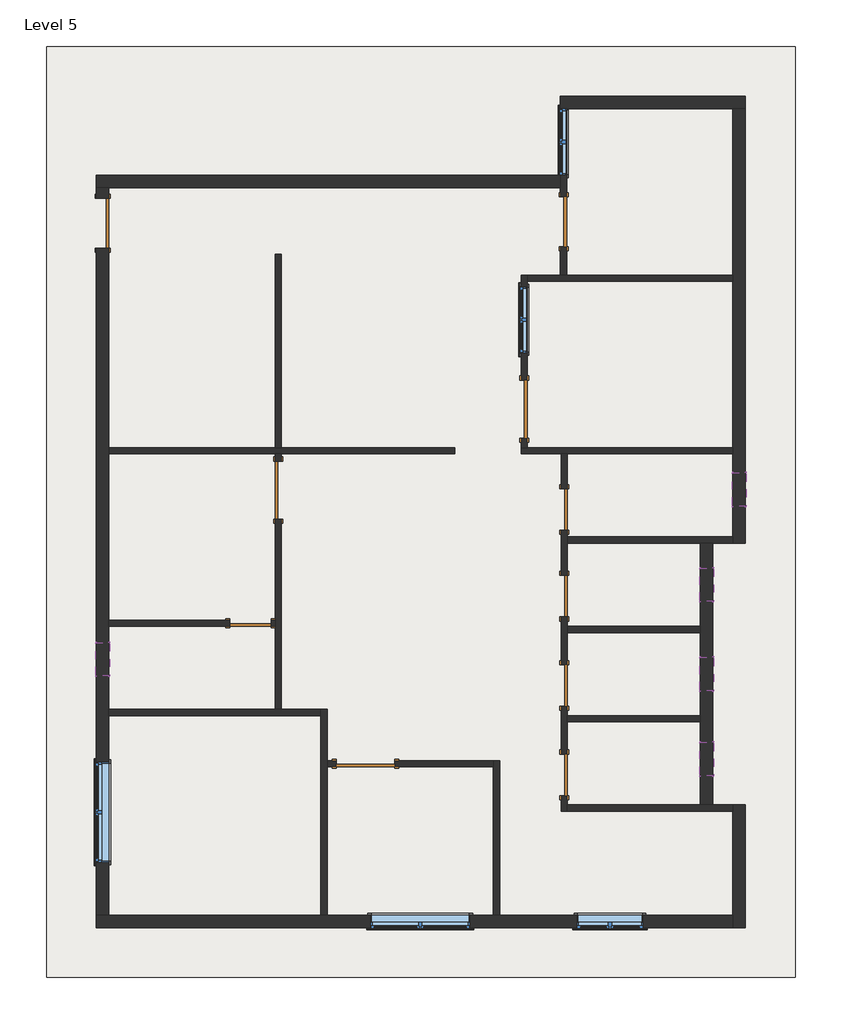
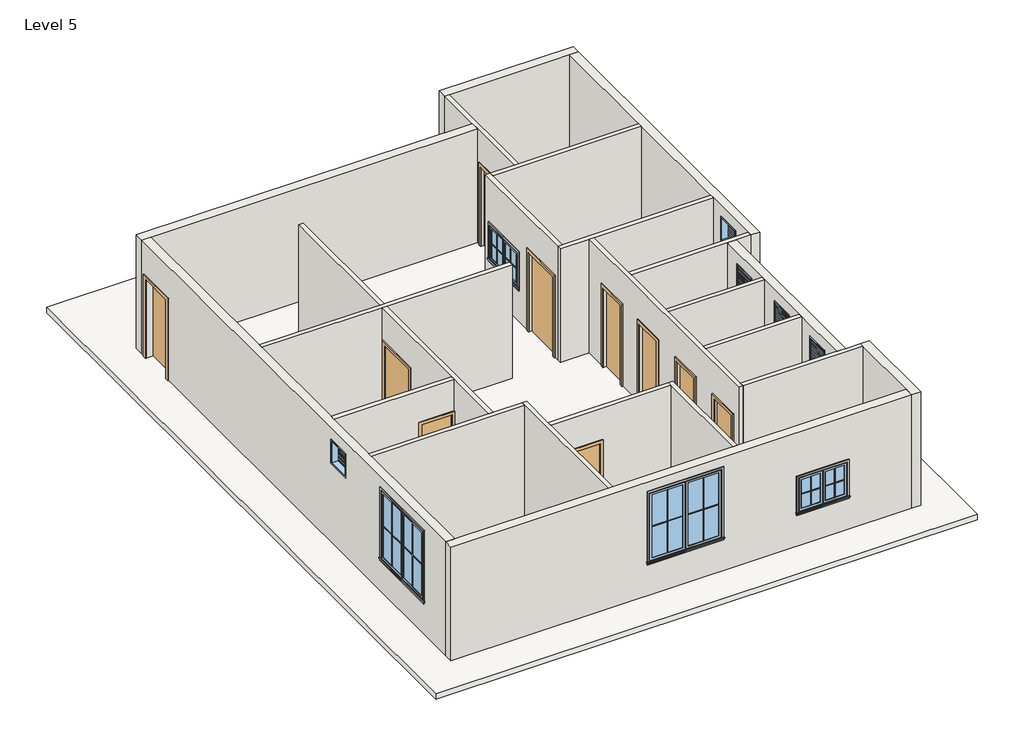
# One storey, incomplete: 23 walls, 20 proxies, 10 doors, 10 windows, 1 roof.
"""IFC4 building model written with IfcOpenShell, lengths in millimetres."""

from ifc_helpers import new_model, si_unit, frame, origin, place, context, project, spatial, polyline, outline, extrude, faceted_brep, transform, mapped, element, save
from components import muntin_pattern_2x2_muntin_pattern_2x2_0a037076, muntin_pattern_2x2_muntin_pattern_2x2_e6f69628, muntin_pattern_2x2_muntin_pattern_2x2_2357e71d, muntin_pattern_2x2_muntin_pattern_2x2_302d8f29, trim_window_exterior_flat_with_sill_b601e94a, trim_window_exterior_flat_with_sill_c4e67c73, trim_window_interior_flat_picture_frame_bfefb25c, trim_window_interior_flat_picture_frame_cf1733af, door_78caadf7, door_214872d5, single_flush_door_3_305aa2a5, single_flush_door_3_a90ba1ad, door_4c162e62, window_casement_double_win_4_c19c33cb, window_casement_double_win_4_2967420f, window_casement_double_win_6_ce442eab, window_f2d8fef0

model = new_model("IFC4")

# Units and contexts
model_context = context("Model", 3, world=origin())
ifc_project = project(units=[si_unit("LENGTHUNIT", "METRE", prefix="MILLI")], contexts=[model_context])

# Site, building, storey
site = spatial("IfcSite", under=ifc_project)
building = spatial("IfcBuilding", under=site)
storey = spatial("IfcBuildingStorey", under=building, Name="Level 5", Elevation=12649.2)

# Proxies
placement = place(None, origin())
muntin_pattern_2x2_muntin_pattern_2x2_shape = muntin_pattern_2x2_muntin_pattern_2x2_0a037076(model_context)
element("IfcBuildingElementProxy", 1, Name="Muntin Pattern_2x2 : Muntin Pattern_2x2", ObjectType="Muntin Pattern_2x2 : Muntin Pattern_2x2", at=placement, inside=storey, context=model_context, shape_type="MappedRepresentation", body=[
    mapped(muntin_pattern_2x2_muntin_pattern_2x2_shape, transform((-7058.058853, -4848.517381, 13633.45), x_axis=(0.0, 1.0, 0.0), y_axis=(-1.0, 0.0, 0.0), z_axis=(0.0, 0.0, 1.0))),
])
element("IfcBuildingElementProxy", 2, Name="Muntin Pattern_2x2 : Muntin Pattern_2x2", ObjectType="Muntin Pattern_2x2 : Muntin Pattern_2x2", at=placement, inside=storey, context=model_context, shape_type="MappedRepresentation", body=[
    mapped(muntin_pattern_2x2_muntin_pattern_2x2_shape, transform((-674.721353, -6497.929881, 13633.45), x_axis=(-1.0, 0.0, 0.0), y_axis=(0.0, -1.0, 0.0), z_axis=(0.0, 0.0, 1.0))),
])
muntin_pattern_2x2_muntin_pattern_2x2_2_shape = muntin_pattern_2x2_muntin_pattern_2x2_e6f69628(model_context)
element("IfcBuildingElementProxy", 3, Name="Muntin Pattern_2x2 : Muntin Pattern_2x2", ObjectType="Muntin Pattern_2x2 : Muntin Pattern_2x2", at=placement, inside=storey, context=model_context, shape_type="MappedRepresentation", body=[
    mapped(muntin_pattern_2x2_muntin_pattern_2x2_2_shape, transform((-7058.058853, -3937.292381, 13633.45), x_axis=(0.0, -1.0, 0.0), y_axis=(1.0, 0.0, 0.0), z_axis=(0.0, 0.0, 1.0))),
])
element("IfcBuildingElementProxy", 4, Name="Muntin Pattern_2x2 : Muntin Pattern_2x2", ObjectType="Muntin Pattern_2x2 : Muntin Pattern_2x2", at=placement, inside=storey, context=model_context, shape_type="MappedRepresentation", body=[
    mapped(muntin_pattern_2x2_muntin_pattern_2x2_2_shape, transform((-1585.946353, -6497.929881, 13633.45), x_axis=(1.0, 0.0, 0.0), y_axis=(0.0, 1.0, 0.0), z_axis=(0.0, 0.0, 1.0))),
])
muntin_pattern_2x2_muntin_pattern_2x2_3_shape = muntin_pattern_2x2_muntin_pattern_2x2_2357e71d(model_context)
element("IfcBuildingElementProxy", 5, Name="Muntin Pattern_2x2 : Muntin Pattern_2x2", ObjectType="Muntin Pattern_2x2 : Muntin Pattern_2x2", at=placement, inside=storey, context=model_context, shape_type="MappedRepresentation", body=[
    mapped(muntin_pattern_2x2_muntin_pattern_2x2_3_shape, transform((2652.678647, -6497.929881, 13633.45), x_axis=(-1.0, 0.0, 0.0), y_axis=(0.0, -1.0, 0.0), z_axis=(0.0, 0.0, 1.0))),
])
element("IfcBuildingElementProxy", 6, Name="Muntin Pattern_2x2 : Muntin Pattern_2x2", ObjectType="Muntin Pattern_2x2 : Muntin Pattern_2x2", at=placement, inside=storey, context=model_context, shape_type="MappedRepresentation", body=[
    mapped(muntin_pattern_2x2_muntin_pattern_2x2_3_shape, transform((727.041147, 4333.582619, 13633.45), x_axis=(0.0, 1.0, 0.0), y_axis=(-1.0, 0.0, 0.0), z_axis=(0.0, 0.0, 1.0))),
])
element("IfcBuildingElementProxy", 7, Name="Muntin Pattern_2x2 : Muntin Pattern_2x2", ObjectType="Muntin Pattern_2x2 : Muntin Pattern_2x2", at=placement, inside=storey, context=model_context, shape_type="MappedRepresentation", body=[
    mapped(muntin_pattern_2x2_muntin_pattern_2x2_3_shape, transform((1450.941147, 7591.132619, 13633.45), x_axis=(0.0, 1.0, 0.0), y_axis=(-1.0, 0.0, 0.0), z_axis=(0.0, 0.0, 1.0))),
])
muntin_pattern_2x2_muntin_pattern_2x2_4_shape = muntin_pattern_2x2_muntin_pattern_2x2_302d8f29(model_context)
element("IfcBuildingElementProxy", 8, Name="Muntin Pattern_2x2 : Muntin Pattern_2x2", ObjectType="Muntin Pattern_2x2 : Muntin Pattern_2x2", at=placement, inside=storey, context=model_context, shape_type="MappedRepresentation", body=[
    mapped(muntin_pattern_2x2_muntin_pattern_2x2_4_shape, transform((2046.253647, -6497.929881, 13633.45), x_axis=(1.0, 0.0, 0.0), y_axis=(0.0, 1.0, 0.0), z_axis=(0.0, 0.0, 1.0))),
])
element("IfcBuildingElementProxy", 9, Name="Muntin Pattern_2x2 : Muntin Pattern_2x2", ObjectType="Muntin Pattern_2x2 : Muntin Pattern_2x2", at=placement, inside=storey, context=model_context, shape_type="MappedRepresentation", body=[
    mapped(muntin_pattern_2x2_muntin_pattern_2x2_4_shape, transform((727.041147, 4940.007619, 13633.45), x_axis=(0.0, -1.0, 0.0), y_axis=(1.0, 0.0, 0.0), z_axis=(0.0, 0.0, 1.0))),
])
element("IfcBuildingElementProxy", 10, Name="Muntin Pattern_2x2 : Muntin Pattern_2x2", ObjectType="Muntin Pattern_2x2 : Muntin Pattern_2x2", at=placement, inside=storey, context=model_context, shape_type="MappedRepresentation", body=[
    mapped(muntin_pattern_2x2_muntin_pattern_2x2_4_shape, transform((1450.941147, 8197.557619, 13633.45), x_axis=(0.0, -1.0, 0.0), y_axis=(1.0, 0.0, 0.0), z_axis=(0.0, 0.0, 1.0))),
])
trim_window_exterior_flat_with_sill_shape = trim_window_exterior_flat_with_sill_b601e94a(model_context)
element("IfcBuildingElementProxy", 11, Name="Trim-Window-Exterior-Flat : with Sill", ObjectType="Trim-Window-Exterior-Flat : with Sill", at=placement, inside=storey, context=model_context, shape_type="MappedRepresentation", body=[
    mapped(trim_window_exterior_flat_with_sill_shape, transform((-7067.583853, -4392.904881, 15392.4), x_axis=(0.0, -1.0, 0.0), y_axis=(0.0, 0.0, 1.0), z_axis=(-1.0, 0.0, 0.0))),
])
element("IfcBuildingElementProxy", 12, Name="Trim-Window-Exterior-Flat : with Sill", ObjectType="Trim-Window-Exterior-Flat : with Sill", at=placement, inside=storey, context=model_context, shape_type="MappedRepresentation", body=[
    mapped(trim_window_exterior_flat_with_sill_shape, transform((-1130.333853, -6507.454881, 15392.4), x_axis=(1.0, 0.0, 0.0), y_axis=(0.0, 0.0, 1.0), z_axis=(0.0, -1.0, 0.0))),
])
trim_window_exterior_flat_with_sill_2_shape = trim_window_exterior_flat_with_sill_c4e67c73(model_context)
element("IfcBuildingElementProxy", 13, Name="Trim-Window-Exterior-Flat : with Sill", ObjectType="Trim-Window-Exterior-Flat : with Sill", at=placement, inside=storey, context=model_context, shape_type="MappedRepresentation", body=[
    mapped(trim_window_exterior_flat_with_sill_2_shape, transform((2349.466147, -6507.454881, 14478.0), x_axis=(1.0, 0.0, 0.0), y_axis=(0.0, 0.0, 1.0), z_axis=(0.0, -1.0, 0.0))),
])
element("IfcBuildingElementProxy", 14, Name="Trim-Window-Exterior-Flat : with Sill", ObjectType="Trim-Window-Exterior-Flat : with Sill", at=placement, inside=storey, context=model_context, shape_type="MappedRepresentation", body=[
    mapped(trim_window_exterior_flat_with_sill_2_shape, transform((717.516147, 4636.795119, 14478.0), x_axis=(0.0, -1.0, 0.0), y_axis=(0.0, 0.0, 1.0), z_axis=(-1.0, 0.0, 0.0))),
])
element("IfcBuildingElementProxy", 15, Name="Trim-Window-Exterior-Flat : with Sill", ObjectType="Trim-Window-Exterior-Flat : with Sill", at=placement, inside=storey, context=model_context, shape_type="MappedRepresentation", body=[
    mapped(trim_window_exterior_flat_with_sill_2_shape, transform((1441.416147, 7894.345119, 14478.0), x_axis=(0.0, -1.0, 0.0), y_axis=(0.0, 0.0, 1.0), z_axis=(-1.0, 0.0, 0.0))),
])
trim_window_interior_flat_picture_frame_shape = trim_window_interior_flat_picture_frame_bfefb25c(model_context)
element("IfcBuildingElementProxy", 16, Name="Trim-Window-Interior-Flat : Picture Frame", ObjectType="Trim-Window-Interior-Flat : Picture Frame", at=placement, inside=storey, context=model_context, shape_type="MappedRepresentation", body=[
    mapped(trim_window_interior_flat_picture_frame_shape, transform((-6838.983853, -4392.904881, 15392.4), x_axis=(0.0, 1.0, 0.0), y_axis=(0.0, 0.0, 1.0), z_axis=(1.0, 0.0, 0.0))),
])
element("IfcBuildingElementProxy", 17, Name="Trim-Window-Interior-Flat : Picture Frame", ObjectType="Trim-Window-Interior-Flat : Picture Frame", at=placement, inside=storey, context=model_context, shape_type="MappedRepresentation", body=[
    mapped(trim_window_interior_flat_picture_frame_shape, transform((-1130.333853, -6278.854881, 15392.4), x_axis=(-1.0, 0.0, 0.0), y_axis=(0.0, 0.0, 1.0), z_axis=(0.0, 1.0, 0.0))),
])
trim_window_interior_flat_picture_frame_2_shape = trim_window_interior_flat_picture_frame_cf1733af(model_context)
element("IfcBuildingElementProxy", 18, Name="Trim-Window-Interior-Flat : Picture Frame", ObjectType="Trim-Window-Interior-Flat : Picture Frame", at=placement, inside=storey, context=model_context, shape_type="MappedRepresentation", body=[
    mapped(trim_window_interior_flat_picture_frame_2_shape, transform((2349.466147, -6278.854881, 14478.0), x_axis=(-1.0, 0.0, 0.0), y_axis=(0.0, 0.0, 1.0), z_axis=(0.0, 1.0, 0.0))),
])
element("IfcBuildingElementProxy", 19, Name="Trim-Window-Interior-Flat : Picture Frame", ObjectType="Trim-Window-Interior-Flat : Picture Frame", at=placement, inside=storey, context=model_context, shape_type="MappedRepresentation", body=[
    mapped(trim_window_interior_flat_picture_frame_2_shape, transform((831.816147, 4636.795119, 14478.0), x_axis=(0.0, 1.0, 0.0), y_axis=(0.0, 0.0, 1.0), z_axis=(1.0, 0.0, 0.0))),
])
element("IfcBuildingElementProxy", 20, Name="Trim-Window-Interior-Flat : Picture Frame", ObjectType="Trim-Window-Interior-Flat : Picture Frame", at=placement, inside=storey, context=model_context, shape_type="MappedRepresentation", body=[
    mapped(trim_window_interior_flat_picture_frame_2_shape, transform((1555.716147, 7894.345119, 14478.0), x_axis=(0.0, 1.0, 0.0), y_axis=(0.0, 0.0, 1.0), z_axis=(1.0, 0.0, 0.0))),
])

# Doors
door_shape = door_78caadf7(model_context)
element("IfcDoor", 21, ObjectType="Single-Flush : 2'6\"", at=placement, inside=storey, context=model_context, shape_type="MappedRepresentation", body=[
    mapped(door_shape, transform((-4241.833853, -925.804881, 12649.2), x_axis=(1.0, 0.0, 0.0), y_axis=(0.0, 1.0, 0.0), z_axis=(0.0, 0.0, 1.0))),
])
door_2_shape = door_214872d5(model_context)
element("IfcDoor", 22, ObjectType="Single-Flush : 2'6\"", at=placement, inside=storey, context=model_context, shape_type="MappedRepresentation", body=[
    mapped(door_2_shape, transform((1511.266147, 1156.995119, 12649.2), x_axis=(0.0, -1.0, 0.0), y_axis=(1.0, 0.0, 0.0), z_axis=(0.0, 0.0, 1.0))),
])
element("IfcDoor", 23, ObjectType="Single-Flush : 2'6\"", at=placement, inside=storey, context=model_context, shape_type="MappedRepresentation", body=[
    mapped(door_2_shape, transform((1511.266147, -430.504881, 12649.2), x_axis=(0.0, -1.0, 0.0), y_axis=(1.0, 0.0, 0.0), z_axis=(0.0, 0.0, 1.0))),
])
element("IfcDoor", 24, ObjectType="Single-Flush : 2'6\"", at=placement, inside=storey, context=model_context, shape_type="MappedRepresentation", body=[
    mapped(door_2_shape, transform((1511.266147, -2068.804881, 12649.2), x_axis=(0.0, -1.0, 0.0), y_axis=(1.0, 0.0, 0.0), z_axis=(0.0, 0.0, 1.0))),
])
element("IfcDoor", 25, ObjectType="Single-Flush : 2'6\"", at=placement, inside=storey, context=model_context, shape_type="MappedRepresentation", body=[
    mapped(door_2_shape, transform((1511.266147, -3707.104881, 12649.2), x_axis=(0.0, -1.0, 0.0), y_axis=(1.0, 0.0, 0.0), z_axis=(0.0, 0.0, 1.0))),
])
single_flush_door_3_shape = single_flush_door_3_305aa2a5(model_context)
element("IfcDoor", 26, ObjectType="Single-Flush : DOOR 3'", at=placement, inside=storey, context=model_context, shape_type="MappedRepresentation", body=[
    mapped(single_flush_door_3_shape, transform((1498.566147, 6433.845119, 12649.2), x_axis=(0.0, 1.0, 0.0), y_axis=(-1.0, 0.0, 0.0), z_axis=(0.0, 0.0, 1.0))),
])
single_flush_door_3_2_shape = single_flush_door_3_a90ba1ad(model_context)
element("IfcDoor", 27, ObjectType="Single-Flush : DOOR 3'", at=placement, inside=storey, context=model_context, shape_type="MappedRepresentation", body=[
    mapped(single_flush_door_3_2_shape, transform((-6953.283853, 6408.445119, 12649.2), x_axis=(0.0, 1.0, 0.0), y_axis=(-1.0, 0.0, 0.0), z_axis=(0.0, 0.0, 1.0))),
])
door_3_shape = door_4c162e62(model_context)
element("IfcDoor", 28, ObjectType="Single-Flush : DOOR 3'6\"", at=placement, inside=storey, context=model_context, shape_type="MappedRepresentation", body=[
    mapped(door_3_shape, transform((-3733.833853, 1512.595119, 12649.2), x_axis=(0.0, 1.0, 0.0), y_axis=(-1.0, 0.0, 0.0), z_axis=(0.0, 0.0, 1.0))),
])
element("IfcDoor", 29, ObjectType="Single-Flush : DOOR 3'6\"", at=placement, inside=storey, context=model_context, shape_type="MappedRepresentation", body=[
    mapped(door_3_shape, transform((774.666147, 2998.495119, 12649.2), x_axis=(0.0, -1.0, 0.0), y_axis=(1.0, 0.0, 0.0), z_axis=(0.0, 0.0, 1.0))),
])
element("IfcDoor", 30, ObjectType="Single-Flush : DOOR 3'6\"", at=placement, inside=storey, context=model_context, shape_type="MappedRepresentation", body=[
    mapped(door_3_shape, transform((-2133.633853, -3503.904881, 12649.2), x_axis=(-1.0, 0.0, 0.0), y_axis=(0.0, -1.0, 0.0), z_axis=(0.0, 0.0, 1.0))),
])

# Roof
element("IfcRoof", 31, ObjectType="Generic - 12\"", at=placement, inside=storey, context=model_context, shape_type="SweptSolid", body=[
    extrude(outline(polyline([(-7981.983853, 9646.945119), (5746.716147, 9646.945119), (5746.716147, -7421.854881), (-7981.983853, -7421.854881), (-7981.983853, 9646.945119)])), frame((0.0, 0.0, 12496.8), z_axis=(0.0, 0.0, 1.0), x_axis=(1.0, 0.0, 0.0)), (0.0, 0.0, 1.0), 152.4),
])

# Walls
element("IfcWall", 32, ObjectType="WALL 4.5\"", at=placement, inside=storey, context=model_context, shape_type="Brep", body=[
    faceted_brep([(-6838.983853, 2179.345119, 12649.2), (-3790.983853, 2179.345119, 12649.2), (-3676.683853, 2179.345119, 12649.2), (-501.683853, 2179.345119, 12649.2), (-501.683853, 2179.345119, 15697.2), (-3676.683853, 2179.345119, 15697.2), (-3790.983853, 2179.345119, 15697.2), (-6838.983853, 2179.345119, 15697.2), (-6838.983853, 2293.645119, 12649.2), (-6838.983853, 2293.645119, 15697.2), (-3790.983853, 2293.645119, 15697.2), (-3676.683853, 2293.645119, 15697.2), (-501.683853, 2293.645119, 15697.2), (-501.683853, 2293.645119, 12649.2), (-3676.683853, 2293.645119, 12649.2), (-3790.983853, 2293.645119, 12649.2)], [[[0, 1, 2, 3, 4, 5, 6, 7]], [[8, 9, 10, 11, 12, 13, 14, 15]], [[3, 2, 1, 0, 8, 15, 14, 13]], [[4, 3, 13, 12]], [[0, 7, 9, 8]], [[7, 6, 5, 4, 12, 11, 10, 9]]]),
])
element("IfcWall", 33, ObjectType="WALL 4.5\"", at=placement, inside=storey, context=model_context, shape_type="Brep", body=[
    faceted_brep([(-2838.483853, -6278.854881, 12649.2), (-2838.483853, -3561.054881, 12649.2), (-2838.483853, -3446.754881, 12649.2), (-2838.483853, -2506.954881, 12649.2), (-2838.483853, -2506.954881, 15697.2), (-2838.483853, -3446.754881, 15697.2), (-2838.483853, -3561.054881, 15697.2), (-2838.483853, -6278.854881, 15697.2), (-2952.783853, -6278.854881, 12649.2), (-2952.783853, -6278.854881, 15697.2), (-2952.783853, -2621.254881, 15697.2), (-2952.783853, -2506.954881, 15697.2), (-2952.783853, -2506.954881, 12649.2), (-2952.783853, -2621.254881, 12649.2)], [[[0, 1, 2, 3, 4, 5, 6, 7]], [[8, 9, 10, 11, 12, 13]], [[3, 2, 1, 0, 8, 13, 12]], [[0, 7, 9, 8]], [[4, 3, 12, 11]], [[7, 6, 5, 4, 11, 10, 9]]]),
])
element("IfcWall", 34, ObjectType="WALL 4.5\"", at=placement, inside=storey, context=model_context, shape_type="Brep", body=[
    faceted_brep([(-2952.783853, -2506.954881, 12649.2), (-3676.683853, -2506.954881, 12649.2), (-3790.983853, -2506.954881, 12649.2), (-6838.983853, -2506.954881, 12649.2), (-6838.983853, -2506.954881, 15697.2), (-3790.983853, -2506.954881, 15697.2), (-3676.683853, -2506.954881, 15697.2), (-2952.783853, -2506.954881, 15697.2), (-2952.783853, -2621.254881, 12649.2), (-2952.783853, -2621.254881, 15697.2), (-6838.983853, -2621.254881, 15697.2), (-6838.983853, -2621.254881, 12649.2)], [[[0, 1, 2, 3, 4, 5, 6, 7]], [[8, 9, 10, 11]], [[3, 2, 1, 0, 8, 11]], [[0, 7, 9, 8]], [[4, 3, 11, 10]], [[7, 6, 5, 4, 10, 9]]]),
])
element("IfcWall", 35, ObjectType="WALL 4.5\"", at=placement, inside=storey, context=model_context, shape_type="SweptSolid", body=[
    extrude(outline(polyline([(14782.8, -3860.833853), (12649.2, -3860.833853), (12649.2, -3790.983853), (15697.2, -3790.983853), (15697.2, -6838.983853), (12649.2, -6838.983853), (12649.2, -4622.833853), (14782.8, -4622.833853), (14782.8, -3860.833853)])), frame((0.0, -982.954881, 0.0), z_axis=(0.0, 1.0, 0.0), x_axis=(0.0, 0.0, 1.0)), (0.0, 0.0, 1.0), 114.3),
])
element("IfcWall", 36, ObjectType="WALL 4.5\"", at=placement, inside=storey, context=model_context, shape_type="Brep", body=[
    faceted_brep([(-3676.683853, 5836.945119, 12649.2), (-3676.683853, 5836.945119, 15697.2), (-3676.683853, 2293.645119, 15697.2), (-3676.683853, 2293.645119, 12649.2), (-3790.983853, 5836.945119, 15697.2), (-3790.983853, 5836.945119, 12649.2), (-3790.983853, 2293.645119, 12649.2), (-3790.983853, 2293.645119, 15697.2)], [[[0, 1, 2, 3]], [[4, 5, 6, 7]], [[5, 0, 3, 6]], [[1, 0, 5, 4]], [[3, 2, 7, 6]], [[1, 4, 7, 2]]]),
    faceted_brep([(-3676.683853, -2506.954881, 15697.2), (-3676.683853, -2506.954881, 12649.2), (-3676.683853, 979.195119, 12649.2), (-3676.683853, 979.195119, 14782.8), (-3676.683853, 2045.995119, 14782.8), (-3676.683853, 2045.995119, 12649.2), (-3676.683853, 2179.345119, 12649.2), (-3676.683853, 2179.345119, 15697.2), (-3790.983853, -2506.954881, 12649.2), (-3790.983853, -2506.954881, 15697.2), (-3790.983853, -982.954881, 15697.2), (-3790.983853, -868.654881, 15697.2), (-3790.983853, 2179.345119, 15697.2), (-3790.983853, 2179.345119, 12649.2), (-3790.983853, 2045.995119, 12649.2), (-3790.983853, 2045.995119, 14782.8), (-3790.983853, 979.195119, 14782.8), (-3790.983853, 979.195119, 12649.2), (-3790.983853, -868.654881, 12649.2), (-3790.983853, -982.954881, 12649.2)], [[[0, 1, 2, 3, 4, 5, 6, 7]], [[8, 9, 10, 11, 12, 13, 14, 15, 16, 17, 18, 19]], [[1, 8, 19, 18, 17, 2]], [[5, 14, 13, 6]], [[1, 0, 9, 8]], [[7, 6, 13, 12]], [[15, 14, 5, 4]], [[16, 15, 4, 3]], [[17, 16, 3, 2]], [[9, 0, 7, 12, 11, 10]]]),
])
element("IfcWall", 37, ObjectType="WALL 4.5\"", at=placement, inside=storey, context=model_context, shape_type="Brep", body=[
    faceted_brep([(4603.716147, 2293.645119, 12649.2), (831.816147, 2293.645119, 12649.2), (717.516147, 2293.645119, 12649.2), (717.516147, 2293.645119, 15697.2), (831.816147, 2293.645119, 15697.2), (4603.716147, 2293.645119, 15697.2), (4603.716147, 2179.345119, 12649.2), (4603.716147, 2179.345119, 15697.2), (1568.416147, 2179.345119, 15697.2), (1454.116147, 2179.345119, 15697.2), (717.516147, 2179.345119, 15697.2), (717.516147, 2179.345119, 12649.2), (1454.116147, 2179.345119, 12649.2), (1568.416147, 2179.345119, 12649.2)], [[[0, 1, 2, 3, 4, 5]], [[6, 7, 8, 9, 10, 11, 12, 13]], [[2, 1, 0, 6, 13, 12, 11]], [[0, 5, 7, 6]], [[3, 2, 11, 10]], [[5, 4, 3, 10, 9, 8, 7]]]),
])
element("IfcWall", 38, ObjectType="WALL 4.5\"", at=placement, inside=storey, context=model_context, shape_type="Brep", body=[
    faceted_brep([(831.816147, 2293.645119, 12649.2), (831.816147, 2465.095119, 12649.2), (831.816147, 2465.095119, 14782.8), (831.816147, 3531.895119, 14782.8), (831.816147, 3531.895119, 12649.2), (831.816147, 5341.645119, 12649.2), (831.816147, 5455.945119, 12649.2), (831.816147, 5455.945119, 15697.2), (831.816147, 5341.645119, 15697.2), (831.816147, 2293.645119, 15697.2), (831.816147, 5246.395119, 14478.0), (831.816147, 5246.395119, 13563.6), (831.816147, 4027.195119, 13563.6), (831.816147, 4027.195119, 14478.0), (717.516147, 2465.095119, 14782.8), (717.516147, 2465.095119, 12649.2), (717.516147, 2293.645119, 12649.2), (717.516147, 2293.645119, 15697.2), (717.516147, 5455.945119, 15697.2), (717.516147, 5455.945119, 12649.2), (717.516147, 3531.895119, 12649.2), (717.516147, 3531.895119, 14782.8), (717.516147, 5246.395119, 14478.0), (717.516147, 4027.195119, 14478.0), (717.516147, 4027.195119, 13563.6), (717.516147, 5246.395119, 13563.6)], [[[0, 1, 2, 3, 4, 5, 6, 7, 8, 9], [10, 11, 12, 13]], [[14, 15, 16, 17, 18, 19, 20, 21], [22, 23, 24, 25]], [[20, 19, 6, 5, 4]], [[16, 15, 1, 0]], [[0, 9, 17, 16]], [[7, 6, 19, 18]], [[11, 10, 22, 25]], [[12, 11, 25, 24]], [[13, 12, 24, 23]], [[10, 13, 23, 22]], [[2, 1, 15, 14]], [[3, 2, 14, 21]], [[4, 3, 21, 20]], [[9, 8, 7, 18, 17]]]),
])
element("IfcWall", 39, ObjectType="WALL 4.5\"", at=placement, inside=storey, context=model_context, shape_type="Brep", body=[
    faceted_brep([(831.816147, 5341.645119, 12649.2), (4603.716147, 5341.645119, 12649.2), (4603.716147, 5341.645119, 15697.2), (831.816147, 5341.645119, 15697.2), (831.816147, 5455.945119, 12649.2), (831.816147, 5455.945119, 15697.2), (1441.416147, 5455.945119, 15697.2), (1555.716147, 5455.945119, 15697.2), (4603.716147, 5455.945119, 15697.2), (4603.716147, 5455.945119, 12649.2), (1555.716147, 5455.945119, 12649.2), (1441.416147, 5455.945119, 12649.2)], [[[0, 1, 2, 3]], [[4, 5, 6, 7, 8, 9, 10, 11]], [[1, 0, 4, 11, 10, 9]], [[0, 3, 5, 4]], [[2, 1, 9, 8]], [[3, 2, 8, 7, 6, 5]]]),
])
element("IfcWall", 40, ObjectType="WALL 4.5\"", at=placement, inside=storey, context=model_context, shape_type="Brep", body=[
    faceted_brep([(1555.716147, 6891.045119, 14782.8), (1555.716147, 6891.045119, 12649.2), (1555.716147, 8503.945119, 12649.2), (1555.716147, 8503.945119, 13563.6), (1555.716147, 7284.745119, 13563.6), (1555.716147, 7284.745119, 14478.0), (1555.716147, 8503.945119, 14478.0), (1555.716147, 8503.945119, 15697.2), (1555.716147, 5455.945119, 15697.2), (1555.716147, 5455.945119, 12649.2), (1555.716147, 5976.645119, 12649.2), (1555.716147, 5976.645119, 14782.8), (1441.416147, 8503.945119, 12649.2), (1441.416147, 7284.745119, 12649.2), (1441.416147, 7056.145119, 12649.2), (1441.416147, 6891.045119, 12649.2), (1441.416147, 6891.045119, 14782.8), (1441.416147, 5976.645119, 14782.8), (1441.416147, 5976.645119, 12649.2), (1441.416147, 5455.945119, 12649.2), (1441.416147, 5455.945119, 15697.2), (1441.416147, 7056.145119, 15697.2), (1441.416147, 7284.745119, 15697.2), (1441.416147, 8503.945119, 15697.2), (1441.416147, 8503.945119, 14478.0), (1441.416147, 7284.745119, 14478.0), (1441.416147, 7284.745119, 13563.6), (1441.416147, 8503.945119, 13563.6)], [[[0, 1, 2, 3, 4, 5, 6, 7, 8, 9, 10, 11]], [[12, 13, 14, 15, 16, 17, 18, 19, 20, 21, 22, 23, 24, 25, 26, 27]], [[10, 9, 19, 18]], [[2, 1, 15, 14, 13, 12]], [[24, 23, 7, 6]], [[12, 27, 3, 2]], [[9, 8, 20, 19]], [[4, 3, 27, 26]], [[5, 4, 26, 25]], [[6, 5, 25, 24]], [[16, 15, 1, 0]], [[17, 16, 0, 11]], [[18, 17, 11, 10]], [[8, 7, 23, 22, 21, 20]]]),
])
element("IfcWall", 41, ObjectType="WALL 4.5\"", at=placement, inside=storey, context=model_context, shape_type="Brep", body=[
    faceted_brep([(4603.716147, 655.345119, 12649.2), (1568.416147, 655.345119, 12649.2), (1568.416147, 655.345119, 15697.2), (4603.716147, 655.345119, 15697.2), (4603.716147, 541.045119, 12649.2), (4603.716147, 541.045119, 15697.2), (4235.416147, 541.045119, 15697.2), (4006.816147, 541.045119, 15697.2), (1568.416147, 541.045119, 15697.2), (1568.416147, 541.045119, 12649.2), (4006.816147, 541.045119, 12649.2), (4235.416147, 541.045119, 12649.2)], [[[0, 1, 2, 3]], [[4, 5, 6, 7, 8, 9, 10, 11]], [[1, 0, 4, 11, 10, 9]], [[0, 3, 5, 4]], [[2, 1, 9, 8]], [[3, 2, 8, 7, 6, 5]]]),
])
element("IfcWall", 42, ObjectType="WALL 4.5\"", at=placement, inside=storey, context=model_context, shape_type="Brep", body=[
    faceted_brep([(1454.116147, -4088.104881, 14782.8), (1454.116147, -4088.104881, 12649.2), (1454.116147, -4373.854881, 12649.2), (1454.116147, -4373.854881, 15697.2), (1454.116147, 2179.345119, 15697.2), (1454.116147, 2179.345119, 12649.2), (1454.116147, 1537.995119, 12649.2), (1454.116147, 1537.995119, 14782.8), (1454.116147, 775.995119, 14782.8), (1454.116147, 775.995119, 12649.2), (1454.116147, -49.504881, 12649.2), (1454.116147, -49.504881, 14782.8), (1454.116147, -811.504881, 14782.8), (1454.116147, -811.504881, 12649.2), (1454.116147, -1687.804881, 12649.2), (1454.116147, -1687.804881, 14782.8), (1454.116147, -2449.804881, 14782.8), (1454.116147, -2449.804881, 12649.2), (1454.116147, -3326.104881, 12649.2), (1454.116147, -3326.104881, 14782.8), (1568.416147, -4373.854881, 12649.2), (1568.416147, -4259.554881, 12649.2), (1568.416147, -4088.104881, 12649.2), (1568.416147, -4088.104881, 14782.8), (1568.416147, -3326.104881, 14782.8), (1568.416147, -3326.104881, 12649.2), (1568.416147, -2735.554881, 12649.2), (1568.416147, -2621.254881, 12649.2), (1568.416147, -2449.804881, 12649.2), (1568.416147, -2449.804881, 14782.8), (1568.416147, -1687.804881, 14782.8), (1568.416147, -1687.804881, 12649.2), (1568.416147, -1097.254881, 12649.2), (1568.416147, -982.954881, 12649.2), (1568.416147, -811.504881, 12649.2), (1568.416147, -811.504881, 14782.8), (1568.416147, -49.504881, 14782.8), (1568.416147, -49.504881, 12649.2), (1568.416147, 541.045119, 12649.2), (1568.416147, 655.345119, 12649.2), (1568.416147, 775.995119, 12649.2), (1568.416147, 775.995119, 14782.8), (1568.416147, 1537.995119, 14782.8), (1568.416147, 1537.995119, 12649.2), (1568.416147, 2179.345119, 12649.2), (1568.416147, 2179.345119, 15697.2), (1568.416147, 655.345119, 15697.2), (1568.416147, 541.045119, 15697.2), (1568.416147, -982.954881, 15697.2), (1568.416147, -1097.254881, 15697.2), (1568.416147, -2621.254881, 15697.2), (1568.416147, -2735.554881, 15697.2), (1568.416147, -4259.554881, 15697.2), (1568.416147, -4373.854881, 15697.2)], [[[0, 1, 2, 3, 4, 5, 6, 7, 8, 9, 10, 11, 12, 13, 14, 15, 16, 17, 18, 19]], [[20, 21, 22, 23, 24, 25, 26, 27, 28, 29, 30, 31, 32, 33, 34, 35, 36, 37, 38, 39, 40, 41, 42, 43, 44, 45, 46, 47, 48, 49, 50, 51, 52, 53]], [[6, 5, 44, 43]], [[10, 9, 40, 39, 38, 37]], [[14, 13, 34, 33, 32, 31]], [[18, 17, 28, 27, 26, 25]], [[2, 1, 22, 21, 20]], [[5, 4, 45, 44]], [[3, 2, 20, 53]], [[41, 40, 9, 8]], [[42, 41, 8, 7]], [[43, 42, 7, 6]], [[35, 34, 13, 12]], [[36, 35, 12, 11]], [[37, 36, 11, 10]], [[29, 28, 17, 16]], [[30, 29, 16, 15]], [[31, 30, 15, 14]], [[23, 22, 1, 0]], [[24, 23, 0, 19]], [[25, 24, 19, 18]], [[4, 3, 53, 52, 51, 50, 49, 48, 47, 46, 45]]]),
])
element("IfcWall", 43, ObjectType="WALL 4.5\"", at=placement, inside=storey, context=model_context, shape_type="Brep", body=[
    faceted_brep([(1568.416147, -4373.854881, 12649.2), (4603.716147, -4373.854881, 12649.2), (4603.716147, -4373.854881, 15697.2), (1568.416147, -4373.854881, 15697.2), (1568.416147, -4259.554881, 12649.2), (1568.416147, -4259.554881, 15697.2), (4006.816147, -4259.554881, 15697.2), (4235.416147, -4259.554881, 15697.2), (4603.716147, -4259.554881, 15697.2), (4603.716147, -4259.554881, 12649.2), (4235.416147, -4259.554881, 12649.2), (4006.816147, -4259.554881, 12649.2)], [[[0, 1, 2, 3]], [[4, 5, 6, 7, 8, 9, 10, 11]], [[1, 0, 4, 11, 10, 9]], [[0, 3, 5, 4]], [[2, 1, 9, 8]], [[3, 2, 8, 7, 6, 5]]]),
])
element("IfcWall", 44, ObjectType="WALL 4.5\"", at=placement, inside=storey, context=model_context, shape_type="SweptSolid", body=[
    extrude(outline(polyline([(4006.816147, -2735.554881), (1568.416147, -2735.554881), (1568.416147, -2621.254881), (4006.816147, -2621.254881), (4006.816147, -2735.554881)])), frame((0.0, 0.0, 12649.2), z_axis=(0.0, 0.0, 1.0), x_axis=(1.0, 0.0, 0.0)), (0.0, 0.0, 1.0), 3048.0),
])
element("IfcWall", 45, ObjectType="WALL 4.5\"", at=placement, inside=storey, context=model_context, shape_type="SweptSolid", body=[
    extrude(outline(polyline([(4006.816147, -1097.254881), (1568.416147, -1097.254881), (1568.416147, -982.954881), (4006.816147, -982.954881), (4006.816147, -1097.254881)])), frame((0.0, 0.0, 12649.2), z_axis=(0.0, 0.0, 1.0), x_axis=(1.0, 0.0, 0.0)), (0.0, 0.0, 1.0), 3048.0),
])
element("IfcWall", 46, ObjectType="WALL 4.5\"", at=placement, inside=storey, context=model_context, shape_type="Brep", body=[
    faceted_brep([(323.816147, -6278.854881, 12649.2), (323.816147, -3446.754881, 12649.2), (323.816147, -3446.754881, 15697.2), (323.816147, -6278.854881, 15697.2), (209.516147, -6278.854881, 12649.2), (209.516147, -6278.854881, 15697.2), (209.516147, -3561.054881, 15697.2), (209.516147, -3446.754881, 15697.2), (209.516147, -3446.754881, 12649.2), (209.516147, -3561.054881, 12649.2)], [[[0, 1, 2, 3]], [[4, 5, 6, 7, 8, 9]], [[1, 0, 4, 9, 8]], [[0, 3, 5, 4]], [[2, 1, 8, 7]], [[3, 2, 7, 6, 5]]]),
])
element("IfcWall", 47, ObjectType="WALL 4.5\"", at=placement, inside=storey, context=model_context, shape_type="SweptSolid", body=[
    extrude(outline(polyline([(12649.2, -2838.483853), (12649.2, -2667.033853), (14782.8, -2667.033853), (14782.8, -1600.233853), (12649.2, -1600.233853), (12649.2, 209.516147), (15697.2, 209.516147), (15697.2, -2838.483853), (12649.2, -2838.483853)])), frame((0.0, -3561.054881, 0.0), z_axis=(0.0, 1.0, 0.0), x_axis=(0.0, 0.0, 1.0)), (0.0, 0.0, 1.0), 114.3),
])
element("IfcWall", 48, ObjectType="WALL 9\"", at=placement, inside=storey, context=model_context, shape_type="Brep", body=[
    faceted_brep([(-7067.583853, 7056.145119, 12649.2), (-6838.983853, 7056.145119, 12649.2), (1441.416147, 7056.145119, 12649.2), (1441.416147, 7056.145119, 15697.2), (-6838.983853, 7056.145119, 15697.2), (-7067.583853, 7056.145119, 15697.2), (-7067.583853, 7284.745119, 12649.2), (-7067.583853, 7284.745119, 15697.2), (1441.416147, 7284.745119, 15697.2), (1441.416147, 7284.745119, 12649.2)], [[[0, 1, 2, 3, 4, 5]], [[6, 7, 8, 9]], [[2, 1, 0, 6, 9]], [[0, 5, 7, 6]], [[3, 2, 9, 8]], [[5, 4, 3, 8, 7]]]),
])
element("IfcWall", 49, ObjectType="WALL 9\"", at=placement, inside=storey, context=model_context, shape_type="Brep", body=[
    faceted_brep([(1441.416147, 8503.945119, 12649.2), (1555.716147, 8503.945119, 12649.2), (4603.716147, 8503.945119, 12649.2), (4832.316147, 8503.945119, 12649.2), (4832.316147, 8503.945119, 15697.2), (4603.716147, 8503.945119, 15697.2), (1555.716147, 8503.945119, 15697.2), (1441.416147, 8503.945119, 15697.2), (1441.416147, 8503.945119, 14478.0), (1441.416147, 8503.945119, 13563.6), (1441.416147, 8732.545119, 12649.2), (1441.416147, 8732.545119, 15697.2), (4832.316147, 8732.545119, 15697.2), (4832.316147, 8732.545119, 12649.2)], [[[0, 1, 2, 3, 4, 5, 6, 7, 8, 9]], [[10, 11, 12, 13]], [[3, 2, 1, 0, 10, 13]], [[4, 3, 13, 12]], [[0, 9, 8, 7, 11, 10]], [[7, 6, 5, 4, 12, 11]]]),
])
element("IfcWall", 50, ObjectType="WALL 9\"", at=placement, inside=storey, context=model_context, shape_type="Brep", body=[
    faceted_brep([(4603.716147, 8503.945119, 12649.2), (4603.716147, 5455.945119, 12649.2), (4603.716147, 5341.645119, 12649.2), (4603.716147, 2293.645119, 12649.2), (4603.716147, 2179.345119, 12649.2), (4603.716147, 655.345119, 12649.2), (4603.716147, 541.045119, 12649.2), (4603.716147, 541.045119, 15697.2), (4603.716147, 655.345119, 15697.2), (4603.716147, 2179.345119, 15697.2), (4603.716147, 2293.645119, 15697.2), (4603.716147, 5341.645119, 15697.2), (4603.716147, 5455.945119, 15697.2), (4603.716147, 8503.945119, 15697.2), (4603.716147, 1830.095119, 15392.4), (4603.716147, 1220.495119, 15392.4), (4603.716147, 1220.495119, 14782.8), (4603.716147, 1830.095119, 14782.8), (4832.316147, 8503.945119, 12649.2), (4832.316147, 8503.945119, 15697.2), (4832.316147, 541.045119, 15697.2), (4832.316147, 541.045119, 12649.2), (4832.316147, 1830.095119, 15392.4), (4832.316147, 1830.095119, 14782.8), (4832.316147, 1220.495119, 14782.8), (4832.316147, 1220.495119, 15392.4)], [[[0, 1, 2, 3, 4, 5, 6, 7, 8, 9, 10, 11, 12, 13], [14, 15, 16, 17]], [[18, 19, 20, 21], [22, 23, 24, 25]], [[6, 5, 4, 3, 2, 1, 0, 18, 21]], [[0, 13, 19, 18]], [[7, 6, 21, 20]], [[23, 22, 14, 17]], [[24, 23, 17, 16]], [[25, 24, 16, 15]], [[22, 25, 15, 14]], [[13, 12, 11, 10, 9, 8, 7, 20, 19]]]),
])
element("IfcWall", 51, ObjectType="WALL 9\"", at=placement, inside=storey, context=model_context, shape_type="Brep", body=[
    faceted_brep([(4006.816147, 541.045119, 12649.2), (4006.816147, -982.954881, 12649.2), (4006.816147, -1097.254881, 12649.2), (4006.816147, -2621.254881, 12649.2), (4006.816147, -2735.554881, 12649.2), (4006.816147, -4259.554881, 12649.2), (4006.816147, -4259.554881, 15697.2), (4006.816147, -2735.554881, 15697.2), (4006.816147, -2621.254881, 15697.2), (4006.816147, -1097.254881, 15697.2), (4006.816147, -982.954881, 15697.2), (4006.816147, 541.045119, 15697.2), (4006.816147, -525.754881, 15392.4), (4006.816147, -525.754881, 14782.8), (4006.816147, 83.845119, 14782.8), (4006.816147, 83.845119, 15392.4), (4006.816147, -2164.054881, 15392.4), (4006.816147, -2164.054881, 14782.8), (4006.816147, -1554.454881, 14782.8), (4006.816147, -1554.454881, 15392.4), (4006.816147, -3719.804881, 15392.4), (4006.816147, -3719.804881, 14782.8), (4006.816147, -3110.204881, 14782.8), (4006.816147, -3110.204881, 15392.4), (4235.416147, 541.045119, 12649.2), (4235.416147, 541.045119, 15697.2), (4235.416147, -4259.554881, 15697.2), (4235.416147, -4259.554881, 12649.2), (4235.416147, -525.754881, 15392.4), (4235.416147, 83.845119, 15392.4), (4235.416147, 83.845119, 14782.8), (4235.416147, -525.754881, 14782.8), (4235.416147, -2164.054881, 15392.4), (4235.416147, -1554.454881, 15392.4), (4235.416147, -1554.454881, 14782.8), (4235.416147, -2164.054881, 14782.8), (4235.416147, -3719.804881, 15392.4), (4235.416147, -3110.204881, 15392.4), (4235.416147, -3110.204881, 14782.8), (4235.416147, -3719.804881, 14782.8)], [[[0, 1, 2, 3, 4, 5, 6, 7, 8, 9, 10, 11], [12, 13, 14, 15], [16, 17, 18, 19], [20, 21, 22, 23]], [[24, 25, 26, 27], [28, 29, 30, 31], [32, 33, 34, 35], [36, 37, 38, 39]], [[5, 4, 3, 2, 1, 0, 24, 27]], [[0, 11, 25, 24]], [[6, 5, 27, 26]], [[13, 12, 28, 31]], [[14, 13, 31, 30]], [[15, 14, 30, 29]], [[12, 15, 29, 28]], [[17, 16, 32, 35]], [[18, 17, 35, 34]], [[19, 18, 34, 33]], [[16, 19, 33, 32]], [[21, 20, 36, 39]], [[22, 21, 39, 38]], [[23, 22, 38, 37]], [[20, 23, 37, 36]], [[11, 10, 9, 8, 7, 6, 26, 25]]]),
])
element("IfcWall", 52, ObjectType="WALL 9\"", at=placement, inside=storey, context=model_context, shape_type="Brep", body=[
    faceted_brep([(4603.716147, -4259.554881, 12649.2), (4603.716147, -4373.854881, 12649.2), (4603.716147, -6278.854881, 12649.2), (4603.716147, -6507.454881, 12649.2), (4603.716147, -6507.454881, 15697.2), (4603.716147, -6278.854881, 15697.2), (4603.716147, -4373.854881, 15697.2), (4603.716147, -4259.554881, 15697.2), (4832.316147, -4259.554881, 12649.2), (4832.316147, -4259.554881, 15697.2), (4832.316147, -6507.454881, 15697.2), (4832.316147, -6507.454881, 12649.2)], [[[0, 1, 2, 3, 4, 5, 6, 7]], [[8, 9, 10, 11]], [[3, 2, 1, 0, 8, 11]], [[4, 3, 11, 10]], [[0, 7, 9, 8]], [[7, 6, 5, 4, 10, 9]]]),
])
element("IfcWall", 53, ObjectType="WALL 9\"", at=placement, inside=storey, context=model_context, shape_type="Brep", body=[
    faceted_brep([(4603.716147, -6278.854881, 12649.2), (323.816147, -6278.854881, 12649.2), (209.516147, -6278.854881, 12649.2), (-2838.483853, -6278.854881, 12649.2), (-2952.783853, -6278.854881, 12649.2), (-6838.983853, -6278.854881, 12649.2), (-7067.583853, -6278.854881, 12649.2), (-7067.583853, -6278.854881, 15697.2), (-6838.983853, -6278.854881, 15697.2), (-2952.783853, -6278.854881, 15697.2), (-2838.483853, -6278.854881, 15697.2), (209.516147, -6278.854881, 15697.2), (323.816147, -6278.854881, 15697.2), (4603.716147, -6278.854881, 15697.2), (-2044.733853, -6278.854881, 15392.4), (-2044.733853, -6278.854881, 13563.6), (-215.933853, -6278.854881, 13563.6), (-215.933853, -6278.854881, 15392.4), (1739.866147, -6278.854881, 14478.0), (1739.866147, -6278.854881, 13563.6), (2959.066147, -6278.854881, 13563.6), (2959.066147, -6278.854881, 14478.0), (4603.716147, -6507.454881, 12649.2), (4603.716147, -6507.454881, 15697.2), (-7067.583853, -6507.454881, 15697.2), (-7067.583853, -6507.454881, 12649.2), (-2044.733853, -6507.454881, 15392.4), (-215.933853, -6507.454881, 15392.4), (-215.933853, -6507.454881, 13563.6), (-2044.733853, -6507.454881, 13563.6), (1739.866147, -6507.454881, 14478.0), (2959.066147, -6507.454881, 14478.0), (2959.066147, -6507.454881, 13563.6), (1739.866147, -6507.454881, 13563.6)], [[[0, 1, 2, 3, 4, 5, 6, 7, 8, 9, 10, 11, 12, 13], [14, 15, 16, 17], [18, 19, 20, 21]], [[22, 23, 24, 25], [26, 27, 28, 29], [30, 31, 32, 33]], [[6, 5, 4, 3, 2, 1, 0, 22, 25]], [[0, 13, 23, 22]], [[7, 6, 25, 24]], [[15, 14, 26, 29]], [[16, 15, 29, 28]], [[17, 16, 28, 27]], [[14, 17, 27, 26]], [[19, 18, 30, 33]], [[20, 19, 33, 32]], [[21, 20, 32, 31]], [[18, 21, 31, 30]], [[13, 12, 11, 10, 9, 8, 7, 24, 23]]]),
])
element("IfcWall", 54, ObjectType="WALL 9\"", at=placement, inside=storey, context=model_context, shape_type="Brep", body=[
    faceted_brep([(-6838.983853, 6865.645119, 14782.8), (-6838.983853, 6865.645119, 12649.2), (-6838.983853, 7056.145119, 12649.2), (-6838.983853, 7056.145119, 15697.2), (-6838.983853, 2293.645119, 15697.2), (-6838.983853, 2179.345119, 15697.2), (-6838.983853, -868.654881, 15697.2), (-6838.983853, -982.954881, 15697.2), (-6838.983853, -2506.954881, 15697.2), (-6838.983853, -2621.254881, 15697.2), (-6838.983853, -6278.854881, 15697.2), (-6838.983853, -6278.854881, 12649.2), (-6838.983853, -2621.254881, 12649.2), (-6838.983853, -2506.954881, 12649.2), (-6838.983853, -982.954881, 12649.2), (-6838.983853, -868.654881, 12649.2), (-6838.983853, 2179.345119, 12649.2), (-6838.983853, 2293.645119, 12649.2), (-6838.983853, 5951.245119, 12649.2), (-6838.983853, 5951.245119, 14782.8), (-6838.983853, -3478.504881, 15392.4), (-6838.983853, -3478.504881, 13563.6), (-6838.983853, -5307.304881, 13563.6), (-6838.983853, -5307.304881, 15392.4), (-6838.983853, -1281.404881, 15392.4), (-6838.983853, -1281.404881, 14782.8), (-6838.983853, -1891.004881, 14782.8), (-6838.983853, -1891.004881, 15392.4), (-7067.583853, 7056.145119, 12649.2), (-7067.583853, 6865.645119, 12649.2), (-7067.583853, 6865.645119, 14782.8), (-7067.583853, 5951.245119, 14782.8), (-7067.583853, 5951.245119, 12649.2), (-7067.583853, -6278.854881, 12649.2), (-7067.583853, -6278.854881, 15697.2), (-7067.583853, 7056.145119, 15697.2), (-7067.583853, -3478.504881, 15392.4), (-7067.583853, -5307.304881, 15392.4), (-7067.583853, -5307.304881, 13563.6), (-7067.583853, -3478.504881, 13563.6), (-7067.583853, -1281.404881, 15392.4), (-7067.583853, -1891.004881, 15392.4), (-7067.583853, -1891.004881, 14782.8), (-7067.583853, -1281.404881, 14782.8)], [[[0, 1, 2, 3, 4, 5, 6, 7, 8, 9, 10, 11, 12, 13, 14, 15, 16, 17, 18, 19], [20, 21, 22, 23], [24, 25, 26, 27]], [[28, 29, 30, 31, 32, 33, 34, 35], [36, 37, 38, 39], [40, 41, 42, 43]], [[2, 1, 29, 28]], [[18, 17, 16, 15, 14, 13, 12, 11, 33, 32]], [[11, 10, 34, 33]], [[3, 2, 28, 35]], [[21, 20, 36, 39]], [[22, 21, 39, 38]], [[23, 22, 38, 37]], [[20, 23, 37, 36]], [[25, 24, 40, 43]], [[26, 25, 43, 42]], [[27, 26, 42, 41]], [[24, 27, 41, 40]], [[30, 29, 1, 0]], [[31, 30, 0, 19]], [[32, 31, 19, 18]], [[10, 9, 8, 7, 6, 5, 4, 3, 35, 34]]]),
])

# Windows
window_casement_double_win_4_shape = window_casement_double_win_4_c19c33cb(model_context)
element("IfcWindow", 55, ObjectType="Window-Casement-Double : WIN 4'", at=placement, inside=storey, context=model_context, shape_type="MappedRepresentation", body=[
    mapped(window_casement_double_win_4_shape, transform((2349.466147, -6393.154881, 12649.2), x_axis=(-1.0, 0.0, 0.0), y_axis=(0.0, -1.0, 0.0), z_axis=(0.0, 0.0, 1.0))),
])
window_casement_double_win_4_2_shape = window_casement_double_win_4_2967420f(model_context)
element("IfcWindow", 56, ObjectType="Window-Casement-Double : WIN 4'", at=placement, inside=storey, context=model_context, shape_type="MappedRepresentation", body=[
    mapped(window_casement_double_win_4_2_shape, transform((774.666147, 4636.795119, 12649.2), x_axis=(0.0, 1.0, 0.0), y_axis=(-1.0, 0.0, 0.0), z_axis=(0.0, 0.0, 1.0))),
])
element("IfcWindow", 57, ObjectType="Window-Casement-Double : WIN 4'", at=placement, inside=storey, context=model_context, shape_type="MappedRepresentation", body=[
    mapped(window_casement_double_win_4_2_shape, transform((1498.566147, 7894.345119, 12649.2), x_axis=(0.0, 1.0, 0.0), y_axis=(-1.0, 0.0, 0.0), z_axis=(0.0, 0.0, 1.0))),
])
window_casement_double_win_6_shape = window_casement_double_win_6_ce442eab(model_context)
element("IfcWindow", 58, ObjectType="Window-Casement-Double : WIN 6'", at=placement, inside=storey, context=model_context, shape_type="MappedRepresentation", body=[
    mapped(window_casement_double_win_6_shape, transform((-6953.283853, -4392.904881, 12649.2), x_axis=(0.0, 1.0, 0.0), y_axis=(-1.0, 0.0, 0.0), z_axis=(0.0, 0.0, 1.0))),
])
element("IfcWindow", 59, ObjectType="Window-Casement-Double : WIN 6'", at=placement, inside=storey, context=model_context, shape_type="MappedRepresentation", body=[
    mapped(window_casement_double_win_6_shape, transform((-1130.333853, -6393.154881, 12649.2), x_axis=(-1.0, 0.0, 0.0), y_axis=(0.0, -1.0, 0.0), z_axis=(0.0, 0.0, 1.0))),
])
window_shape = window_f2d8fef0(model_context)
element("IfcWindow", 60, ObjectType="Window-Louvers : 24\" x 24\"", at=placement, inside=storey, context=model_context, shape_type="MappedRepresentation", body=[
    mapped(window_shape, transform((4724.366147, 1525.295119, 13868.4), x_axis=(0.0, -1.0, 0.0), y_axis=(1.0, 0.0, 0.0), z_axis=(0.0, 0.0, 1.0))),
])
element("IfcWindow", 61, ObjectType="Window-Louvers : 24\" x 24\"", at=placement, inside=storey, context=model_context, shape_type="MappedRepresentation", body=[
    mapped(window_shape, transform((4114.766147, -220.954881, 13868.4), x_axis=(0.0, 1.0, 0.0), y_axis=(-1.0, 0.0, 0.0), z_axis=(0.0, 0.0, 1.0))),
])
element("IfcWindow", 62, ObjectType="Window-Louvers : 24\" x 24\"", at=placement, inside=storey, context=model_context, shape_type="MappedRepresentation", body=[
    mapped(window_shape, transform((4114.766147, -1859.254881, 13868.4), x_axis=(0.0, 1.0, 0.0), y_axis=(-1.0, 0.0, 0.0), z_axis=(0.0, 0.0, 1.0))),
])
element("IfcWindow", 63, ObjectType="Window-Louvers : 24\" x 24\"", at=placement, inside=storey, context=model_context, shape_type="MappedRepresentation", body=[
    mapped(window_shape, transform((4114.766147, -3415.004881, 13868.4), x_axis=(0.0, 1.0, 0.0), y_axis=(-1.0, 0.0, 0.0), z_axis=(0.0, 0.0, 1.0))),
])
element("IfcWindow", 64, ObjectType="Window-Louvers : 24\" x 24\"", at=placement, inside=storey, context=model_context, shape_type="MappedRepresentation", body=[
    mapped(window_shape, transform((-6946.933853, -1586.204881, 13868.4), x_axis=(0.0, -1.0, 0.0), y_axis=(1.0, 0.0, 0.0), z_axis=(0.0, 0.0, 1.0))),
])

save(model, "model.ifc")

# Revit data of these elements
# Type "Muntin Pattern_2x2 : Muntin Pattern_2x2"
#   Width [instance default] = 4' - 0"
#   Thickness = 0' - 0 1/2"
#   Height [instance default] = 4' - 0"
#   Distance = 0' - 0 3/4"
#   Interior Material [instance default] = none
#   Exterior Material [instance default] = none
#   Default Elevation = 0
# Type "Trim-Window-Exterior-Flat : with Sill"
#   Trim Width = 0' - 2 1/4"
#   Trim Thickness_Picture Frame = 0' - 1 1/4"
#   Trim Thickness_with Sill = 0' - 0 3/4"
#   Sill Thickness = 0' - 1 1/4"
#   Opening Width [instance default] = 2' - 0"
#   Opening Height [instance default] = 3' - 0"
#   Default Elevation = 4' - 0"
#   Sill = yes
#   Picture Frame = no
#   Trim Material [instance default] = none
# Type "Trim-Window-Interior-Flat : Picture Frame"
#   Trim Thickness_Picture Frame = 0' - 1 1/4"
#   Trim Width = 0' - 2 1/4"
#   Trim Thickness_with Sill = 0' - 0 3/4"
#   Sill Thickness = 0' - 1 1/4"
#   Opening Width [instance default] = 2' - 0"
#   Opening Height [instance default] = 3' - 0"
#   Default Elevation = 4' - 0"
#   Sill = no
#   Picture Frame = yes
#   Trim Material [instance default] = none
# Type "Single-Flush : 2'6\""
#   Type Mark = "10"
#   Construction Type Id = "MDOOR"
#   Assembly Code = "C1020"
#   Analytic Construction = "Metal"
#   Thickness = 0' - 2"
#   Heat Transfer Coefficient (U) = 0.651978 BTU/(h·ft²·°F)
#   Height = 7' - 0"
#   Trim Projection Ext = 0' - 1"
#   Trim Projection Int = 0' - 1"
#   Trim Width = 0' - 3"
#   Width = 2' - 6"
#   Define Thermal Properties by = 1
#   Door Material = Door - Panel
#   Frame Material = Door - Frame
#   Visual Light Transmittance = 0
#   Solar Heat Gain Coefficient = 0
#   Function = (empty or 0)
#   Wall Closure = (empty or 0)
# Type "Single-Flush : DOOR 3'"
#   Type Mark = "8"
#   Construction Type Id = "MDOOR"
#   Assembly Code = "C1020"
#   Analytic Construction = "Metal"
#   Thickness = 0' - 2"
#   Heat Transfer Coefficient (U) = 0.651978 BTU/(h·ft²·°F)
#   Height = 7' - 0"
#   Trim Projection Ext = 0' - 1"
#   Trim Projection Int = 0' - 1"
#   Trim Width = 0' - 3"
#   Width = 3' - 0"
#   Define Thermal Properties by = 1
#   Door Material = Door - Panel
#   Frame Material = Door - Frame
#   Visual Light Transmittance = 0
#   Solar Heat Gain Coefficient = 0
#   Function = (empty or 0)
#   Wall Closure = (empty or 0)
# Type "Single-Flush : DOOR 3'6\""
#   Type Mark = "9"
#   Construction Type Id = "MDOOR"
#   Assembly Code = "C1020"
#   Analytic Construction = "Metal"
#   Thickness = 0' - 2"
#   Heat Transfer Coefficient (U) = 0.651978 BTU/(h·ft²·°F)
#   Height = 7' - 0"
#   Trim Projection Ext = 0' - 1"
#   Trim Projection Int = 0' - 1"
#   Trim Width = 0' - 3"
#   Width = 3' - 6"
#   Define Thermal Properties by = 1
#   Door Material = Door - Panel
#   Frame Material = Door - Frame
#   Visual Light Transmittance = 0
#   Solar Heat Gain Coefficient = 0
#   Function = (empty or 0)
#   Wall Closure = (empty or 0)
# Type "Generic - 12\""
#   Assembly Code = "B1020"
#   Layers, outside or top first: 0' - 6" no material (function 1)
# Type "WALL 4.5\""
#   Assembly Code = "B2010"
#   Layers, outside or top first: 0' - 4 1/2" no material (function 1)
# Type "WALL 9\""
#   Assembly Code = "B2010"
#   Layers, outside or top first: 0' - 9" no material (function 1)
# Type "Window-Casement-Double : WIN 4'"
#   Type Mark = "18"
#   Fire Rating = "0.5h"
#   Assembly Code = "B2020100"
#   Analytic Construction = "Double glazing - domestic"
#   Frame Extension [instance default] = 0' - 0 1/4"
#   Window Inset [instance default] = 0' - 0"
#   Wall Thickness [instance default] = 0' - 6"
#   Interior Wall Closure [instance default] = 0' - 2 1/4"
#   Half Width = 2' - 0"
#   Visual Light Transmittance = 0.81
#   Thermal Resistance (R) = 1.8146 (h·ft²·°F)/BTU
#   Solar Heat Gain Coefficient = 0.76
#   Rough Width = 4' - 0 1/2"
#   Rough Height = 3' - 0 1/2"
#   Height = 3' - 0"
#   Heat Transfer Coefficient (U) = 0.5511 BTU/(h·ft²·°F)
#   Exterior Wall Closure [instance default] = 0' - 1 1/4"
#   Extension Jamb [instance default] = 0' - 2 1/4"
#   Default Sill Height = 3' - 0"
#   Width = 4' - 0"
#   Muntin Visibility = yes
#   Interior Trim Visibility [instance default] = yes
#   Exterior Trim Visibility [instance default] = yes
#   Extension Jamb Visibility [instance default] = yes
#   Interior Trim Material = Wood - Stained
#   Muntin Pattern = Muntin Pattern_2x2 : Muntin Pattern_2x2
#   Interior Trim = Trim-Window-Interior-Flat : Picture Frame
#   Interior Frame Material = Wood - Stained
#   Glass Panel Material = Glass
#   Exterior Trim Material = Clad - White
#   Exterior Trim = Trim-Window-Exterior-Flat : with Sill
#   Exterior Frame Material = Clad - White
#   Wall Closure = (empty or 0)
# Type "Window-Casement-Double : WIN 6'"
#   Type Mark = "19"
#   Fire Rating = "0.5h"
#   Assembly Code = "B2020100"
#   Analytic Construction = "Double glazing - domestic"
#   Frame Extension [instance default] = 0' - 0 1/4"
#   Window Inset [instance default] = 0' - 0"
#   Wall Thickness [instance default] = 0' - 6"
#   Interior Wall Closure [instance default] = 0' - 2 1/4"
#   Half Width = 3' - 0"
#   Visual Light Transmittance = 0.81
#   Thermal Resistance (R) = 1.8146 (h·ft²·°F)/BTU
#   Solar Heat Gain Coefficient = 0.76
#   Rough Width = 6' - 0 1/2"
#   Rough Height = 6' - 0 1/2"
#   Height = 6' - 0"
#   Heat Transfer Coefficient (U) = 0.5511 BTU/(h·ft²·°F)
#   Exterior Wall Closure [instance default] = 0' - 1 1/4"
#   Extension Jamb [instance default] = 0' - 2 1/4"
#   Default Sill Height = 3' - 0"
#   Width = 6' - 0"
#   Muntin Visibility = yes
#   Interior Trim Visibility [instance default] = yes
#   Exterior Trim Visibility [instance default] = yes
#   Extension Jamb Visibility [instance default] = yes
#   Interior Trim Material = Wood - Stained
#   Muntin Pattern = Muntin Pattern_2x2 : Muntin Pattern_2x2
#   Interior Trim = Trim-Window-Interior-Flat : Picture Frame
#   Interior Frame Material = Wood - Stained
#   Glass Panel Material = Glass
#   Exterior Trim Material = Clad - White
#   Exterior Trim = Trim-Window-Exterior-Flat : with Sill
#   Exterior Frame Material = Clad - White
#   Wall Closure = (empty or 0)
# Type "Window-Louvers : 24\" x 24\""
#   Type Mark = "20"
#   Construction Type Id = "GSP4R"
#   Assembly Code = "B20"
#   Analytic Construction = "1/8 in Pilkington single glazing"
#   Visual Light Transmittance = 0.9
#   Thermal Resistance (R) = 1.53941 (h·ft²·°F)/BTU
#   Solar Heat Gain Coefficient = 0.78
#   Max Height = 1' - 11.74264"
#   Height = 2' - 0"
#   Heat Transfer Coefficient (U) = 0.6496 BTU/(h·ft²·°F)
#   Blade Width [instance default] = 1' - 10 1/2"
#   Blade Vertical Thickness = 0' - 0.35355"
#   Blade Thickness = 0' - 0 1/4"
#   Blade Spacing = 0' - 1 1/2"
#   Blade Height = 0' - 1.85355"
#   Blade Depth = 0' - 3"
#   Blade Angle = 45.00°
#   Default Sill Height = 3' - 0"
#   Trim Projection_Exterior = 0' - 0 1/2"
#   Trim Projection_Interior = 0' - 0 1/2"
#   Trim Width_Exterior = 0' - 1 1/2"
#   Trim Width_Interior = 0' - 1 1/2"
#   Width = 2' - 0"
#   Max Blade Count = 12
#   Define Thermal Properties by = 1
#   Blade Count = 12
#   Frame Material = Birch
#   Louver Material = Birch
#   Trim Exterior Material = Birch
#   Trim Interior Material = Birch
#   Wall Closure = (empty or 0)
# Elements 1, 2, 3, 4 (IfcBuildingElementProxy, "Muntin Pattern_2x2 : Muntin Pattern_2x2")
#   Width = 2' - 6 5/8"
#   Height = 5' - 6 1/2"
#   Interior Material = Wood - Stained
#   Exterior Material = Clad - White
#   Phase Created = New Construction
#   Materials on its faces: "Clad - White", "Wood - Stained"
# Elements 5, 6, 7, 8, 9, 10 (IfcBuildingElementProxy, "Muntin Pattern_2x2 : Muntin Pattern_2x2")
#   Width = 1' - 6 5/8"
#   Height = 2' - 6 1/2"
#   Interior Material = Wood - Stained
#   Exterior Material = Clad - White
#   Phase Created = New Construction
#   Materials on its faces: "Clad - White", "Wood - Stained"
# Elements 11, 12 (IfcBuildingElementProxy, "Trim-Window-Exterior-Flat : with Sill")
#   Opening Width = 6' - 0"
#   Opening Height = 6' - 0"
#   Trim Material = Clad - White
#   Phase Created = New Construction
#   Materials on its faces: "Clad - White"
# Elements 13, 14, 15 (IfcBuildingElementProxy, "Trim-Window-Exterior-Flat : with Sill")
#   Opening Width = 4' - 0"
#   Opening Height = 3' - 0"
#   Trim Material = Clad - White
#   Phase Created = New Construction
#   Materials on its faces: "Clad - White"
# Elements 16, 17 (IfcBuildingElementProxy, "Trim-Window-Interior-Flat : Picture Frame")
#   Opening Width = 6' - 0"
#   Opening Height = 6' - 0"
#   Trim Material = Wood - Stained
#   Phase Created = New Construction
#   Materials on its faces: "Wood - Stained"
# Elements 18, 19, 20 (IfcBuildingElementProxy, "Trim-Window-Interior-Flat : Picture Frame")
#   Opening Width = 4' - 0"
#   Opening Height = 3' - 0"
#   Trim Material = Wood - Stained
#   Phase Created = New Construction
#   Materials on its faces: "Wood - Stained"
# Elements 21, 22, 23, 24, 25 (IfcDoor, "Single-Flush : 2'6\"")
#   Phase Created = New Construction
#   Materials on its faces: "Door - Frame", "Door - Panel"
# Elements 26, 27 (IfcDoor, "Single-Flush : DOOR 3'")
#   Phase Created = New Construction
#   Materials on its faces: "Door - Frame", "Door - Panel"
# Elements 28, 29, 30 (IfcDoor, "Single-Flush : DOOR 3'6\"")
#   Phase Created = New Construction
#   Materials on its faces: "Door - Frame", "Door - Panel"
# Element 31 (IfcRoof, "Generic - 12\"")
#   built-in parameter 1001705 = 41.5 (stored number, unit not read)
#   built-in parameter 1001701 = -0.5 (stored number, unit not read)
#   built-in parameter 1001710 = 33615
#   Phase Created = New Construction
#   Materials on its faces: "Default Roof", "Cherry", "Wood Planks"
# Elements 32, 33, 34, 35, 36, 37, 38, 39, 42, 43, 44, 45, 46, 47 (IfcWall, "WALL 4.5\"")
#   Top Offset = 0' - 0"
#   Base Offset = 0' - 0"
#   Unconnected Height = 10' - 0"
#   wall height = 10' - 0"
#   Phase Created = New Construction
#   Base Constraint = Level 5
#   Materials on its faces: "Default Wall"
# Elements 40, 41 (IfcWall, "WALL 4.5\"")
#   Top Offset = 0' - 0"
#   Base Offset = 0' - 0"
#   Unconnected Height = 10' - 0"
#   wall height = 10' - 0"
#   Phase Created = New Construction
#   Base Constraint = Level 5
#   Materials on its faces: "Default Wall", "Wood - Stained"
# Elements 48, 49, 50, 51, 52, 53, 54 (IfcWall, "WALL 9\"")
#   Top Offset = 0' - 0"
